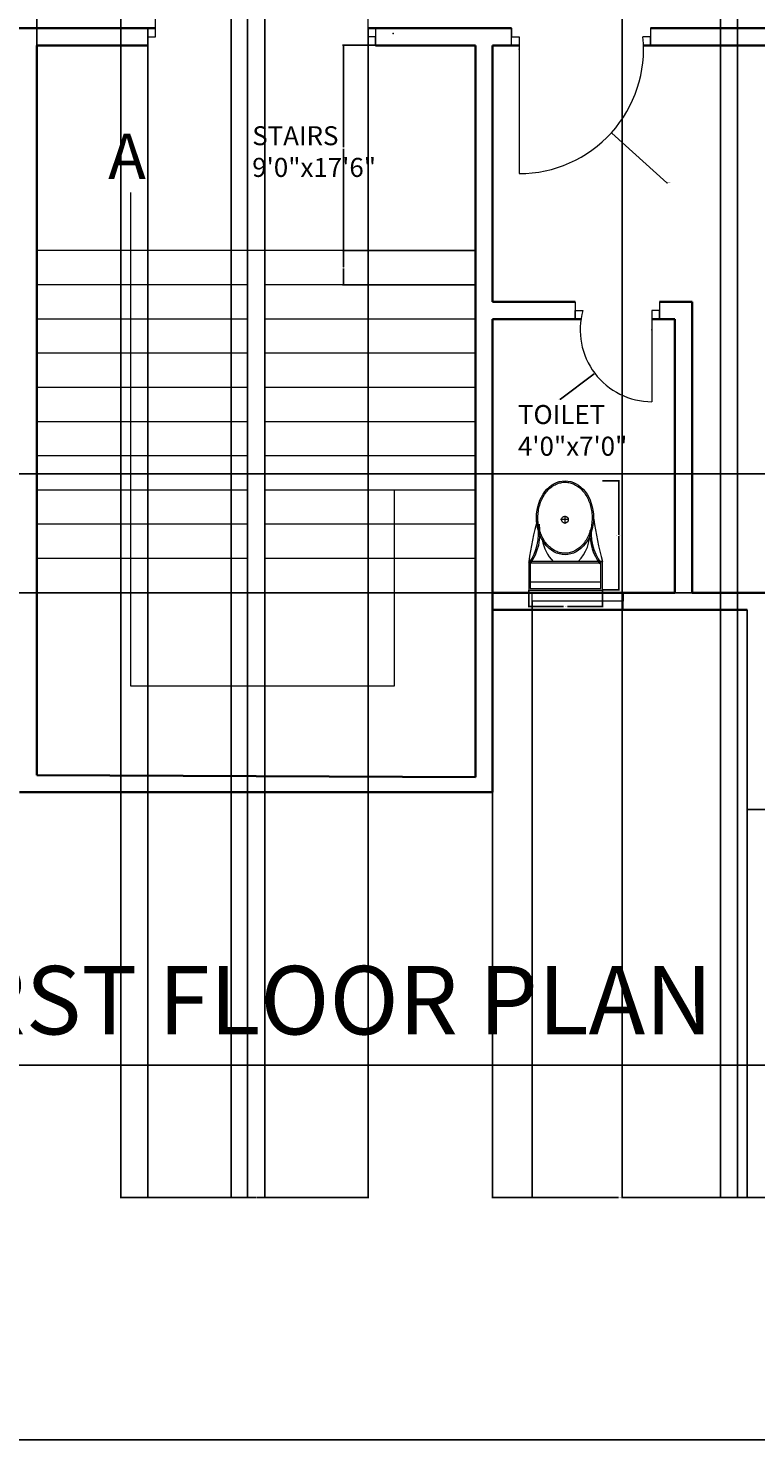
# Model space of a CAD drawing. Units: inches. Extents: x 1861 to 2564, y 1482 to 2317.
# Tile 2 of 11: x 2155 to 2347, y 1482 to 1853. Entities that reach past the tile are written whole.
import ezdxf

# ---------------------------------------------------------------- set-up
doc = ezdxf.new("R2010")
doc.units = ezdxf.units.IN
for name, color, linetype, lineweight in [('A-ANNO-DIMS', 2, 'Continuous', 18), ('A-ANNO-SYMB', 7, 'Continuous', 18), ('A-ANNO-TEXT', 7, 'Continuous', 25), ('A-ANNO-TTLB', 7, 'Continuous', 25), ('A-AREA-IDEN', 7, 'Continuous', 18), ('A-DOOR', 3, 'Continuous', 18), ('A-FLOR-EDGE', 7, 'Continuous', 25), ('A-FLOR-FIXT', 8, 'Continuous', 18), ('A-FLOR-STRS', 7, 'Continuous', 18), ('A-GLAZ', 4, 'Continuous', 18), ('A-WALL', 7, 'Continuous', 35)]:
    doc.layers.add(name, color=color, linetype=linetype, lineweight=lineweight)
doc.styles.get("Standard").update_dxf_attribs({"font": 'arial.ttf'})
doc.dimstyles.get("Standard").update_dxf_attribs({"dimtxt": 0.18, "dimasz": 0.18, "dimexe": 0.18, "dimexo": 0.0625, "dimgap": 0.09, "dimtad": 0, "dimtih": 1, "dimtoh": 1, "dimdec": 4, "dimzin": 0, "dimdsep": 46, "dimtxsty": 'Standard', "dimcen": 0.09, "dimadec": 0, "dimazin": 0, "dimtfac": 1, "dimtdec": 4, "dimtofl": 0, "dimtmove": 0, "dimatfit": 3, "dimfxl": 1, "dimtolj": 1, "dimtzin": 0, "dimarcsym": 0})

# ---------------------------------------------------------------- blocks, each defined once
blk = doc.blocks.new('A$C31115884')
for p, q in [((257.5, 466.4), (257.5, 523.2)), ((283.1, 497.7), (223.4, 497.7)), ((0, 200), (0, 0)), ((520, 200), (0, 200)), ((520, 0), (520, 200)), ((10, 190), (10, 10)), ((510, 190), (10, 190)), ((510, 10), (510, 190)), ((510, 54.5), (0, 54.5)), ((10, 10), (510, 10)), ((0, 0), (520, 0))]:
    blk.add_line(p, q)
blk.add_circle((255.6, 496.4), 23.6)
for centre, radius, start, end in [((2777.7, -204.6), 2807, 165.4549, 171.71327), ((3237, 905), 2807, 188.28673, 194.5451), ((-294.5, 403.3), 364.7, 324.20913, 9.34987), ((-294.5, 403.3), 374.7, 324.20913, 9.34987), ((139.5, 406.2), 293.5, 315.84364, 2.65635), ((805.8, 403.3), 374.7, 179.20365, 215.79087), ((805.8, 403.3), 364.7, 170.65013, 215.79087), ((383.6, 406.2), 293.5, 190.27735, 224.15636)]:
    blk.add_arc(centre, radius, start, end)
blk.add_ellipse((256.2, 509.9), major_axis=(0, -260.7), ratio=0.772727)
blk.add_open_spline([(256.2, 259.2), (263.1, 259.2), (270, 259.7), (287.8, 262.3), (298.7, 265.1), (319.9, 273.1), (330.2, 278.4), (350.1, 291.1), (359.7, 298.7), (377.7, 315.9), (386.2, 325.5), (401.7, 346.6), (408.8, 358.1), (421.3, 382.5), (426.8, 395.5), (435.9, 422.4), (439.5, 436.4), (444.8, 465.1), (446.5, 479.7), (447.9, 509.2), (447.6, 524), (445, 553.3), (442.7, 567.8), (436.3, 596), (432.1, 609.7), (421.9, 636), (416, 648.6), (402.5, 672.1), (395, 683), (378.6, 703), (369.8, 712.1), (351.1, 728), (341.3, 734.8), (320.9, 746.2), (310.4, 750.7), (288.9, 757.3), (278, 759.4), (256, 761), (245, 760.6), (223.1, 757.2), (212.3, 754.3), (191.1, 746.1), (180.8, 740.7), (160.9, 727.8), (151.4, 720.1), (133.5, 702.7), (125.1, 693), (109.6, 671.7), (102.6, 660.2), (90.2, 635.7), (84.9, 622.7), (76, 595.6), (72.4, 581.6), (67.2, 552.9), (65.6, 538.2), (64.4, 508.8), (64.8, 494), (67.5, 464.7), (69.9, 450.2), (76.6, 422), (80.8, 408.3), (91.1, 382.2), (97.2, 369.7), (110.8, 346.3), (118.4, 335.4), (134.8, 315.6), (143.7, 306.7), (162.4, 290.9), (172.3, 284.2), (192.8, 273), (203.3, 268.6), (224.8, 262.2), (235.8, 260.2), (249.9, 259.3), (253, 259.2), (256.2, 259.2)], degree=3, knots=[0, 0, 0, 0, 0.110105, 0.110105, 0.285049, 0.285049, 0.459994, 0.459994, 0.634938, 0.634938, 0.809882, 0.809882, 0.984827, 0.984827, 1.159771, 1.159771, 1.334715, 1.334715, 1.50966, 1.50966, 1.684604, 1.684604, 1.859549, 1.859549, 2.034493, 2.034493, 2.209437, 2.209437, 2.384382, 2.384382, 2.559326, 2.559326, 2.73427, 2.73427, 2.909215, 2.909215, 3.084159, 3.084159, 3.259103, 3.259103, 3.434048, 3.434048, 3.608992, 3.608992, 3.783936, 3.783936, 3.958881, 3.958881, 4.133825, 4.133825, 4.30877, 4.30877, 4.483714, 4.483714, 4.658658, 4.658658, 4.833603, 4.833603, 5.008547, 5.008547, 5.183491, 5.183491, 5.358436, 5.358436, 5.53338, 5.53338, 5.708324, 5.708324, 5.883269, 5.883269, 6.058213, 6.058213, 6.233158, 6.233158, 6.283185, 6.283185, 6.283185, 6.283185])
blk = doc.blocks.new('WIN-24IN')
for p, q in [((0, 24), (4.5, 24)), ((4.5, 24), (2.25, 24)), ((2.25, 24), (2.25, 0)), ((2.25, 0), (0, 0)), ((0, 0), (4.5, 0))]:
    blk.add_line(p, q)
blk = doc.blocks.new('*D14')
at = {"layer": 'A-ANNO-DIMS', "color": 0, "lineweight": -2, "transparency": 16777216}
for p, q in [((2306.19, 1734.33), (2310.61, 1734.33)), ((2310.43, 1734.15), (2310.43, 1720.15)), ((2310.43, 1705.79), (2310.43, 1719.79)), ((2306.19, 1705.61), (2310.61, 1705.61))]:
    blk.add_line(p, q, dxfattribs=at)
at = {"layer": 'A-ANNO-DIMS', "color": 0, "transparency": 16777216}
for points in [[(2310.4, 1734.15), (2310.46, 1734.15), (2310.43, 1734.33)], [(2310.4, 1705.79), (2310.46, 1705.79), (2310.43, 1705.61)]]:
    blk.add_solid(points, dxfattribs=at)
at = {"layer": 'Defpoints', "color": 0, "transparency": 16777216}
for p in [(2306.13, 1734.33), (2310.43, 1734.33), (2306.13, 1705.61)]:
    blk.add_point(p, dxfattribs=at)
at = {"layer": 'A-ANNO-DIMS', "color": 0, "transparency": 16777216, "insert": (2310.43, 1719.97), "char_height": 0.18, "attachment_point": 5}
blk.add_mtext('\\A1;WC 29 TYP.', dxfattribs=at)
blk = doc.blocks.new('*D15')
at = {"layer": 'A-ANNO-DIMS', "color": 0, "lineweight": -2, "transparency": 16777216}
for p, q in [((2286.74, 1705.55), (2286.74, 1701.12)), ((2306.13, 1705.55), (2306.13, 1701.12)), ((2286.92, 1701.3), (2295.92, 1701.3)), ((2305.95, 1701.3), (2296.96, 1701.3))]:
    blk.add_line(p, q, dxfattribs=at)
at = {"layer": 'A-ANNO-DIMS', "color": 0, "transparency": 16777216}
for points in [[(2286.92, 1701.33), (2286.92, 1701.27), (2286.74, 1701.3)], [(2305.95, 1701.33), (2305.95, 1701.27), (2306.13, 1701.3)]]:
    blk.add_solid(points, dxfattribs=at)
at = {"layer": 'Defpoints', "color": 0, "transparency": 16777216}
for p in [(2286.74, 1705.61), (2306.13, 1705.61), (2306.13, 1701.3)]:
    blk.add_point(p, dxfattribs=at)
at = {"layer": 'A-ANNO-DIMS', "color": 0, "transparency": 16777216, "insert": (2296.44, 1701.3), "char_height": 0.18, "attachment_point": 5}
blk.add_mtext('\\A1;19 TYP.', dxfattribs=at)
blk = doc.blocks.new('*D37')
at = {"layer": 'A-ANNO-DIMS', "color": 0, "lineweight": -2, "transparency": 16777216}
for p, q in [((2311.38, 2250.82), (2311.38, 1545.6)), ((2337.24, 2250.82), (2337.24, 1545.6)), ((2311.56, 1545.78), (2323.91, 1545.78)), ((2337.06, 1545.78), (2324.7, 1545.78))]:
    blk.add_line(p, q, dxfattribs=at)
at = {"layer": 'A-ANNO-DIMS', "color": 0, "transparency": 16777216}
for points in [[(2311.56, 1545.81), (2311.56, 1545.75), (2311.38, 1545.78)], [(2337.06, 1545.81), (2337.06, 1545.75), (2337.24, 1545.78)]]:
    blk.add_solid(points, dxfattribs=at)
at = {"layer": 'Defpoints', "color": 0, "transparency": 16777216}
for p in [(2311.38, 2250.89), (2337.24, 2250.89), (2337.24, 1545.78)]:
    blk.add_point(p, dxfattribs=at)
at = {"layer": 'A-ANNO-DIMS', "color": 0, "transparency": 16777216, "insert": (2324.31, 1545.78), "char_height": 0.18, "attachment_point": 5}
blk.add_mtext('\\A1;25.86', dxfattribs=at)
blk = doc.blocks.new('*D38')
at = {"layer": 'A-ANNO-DIMS', "color": 0, "lineweight": -2, "transparency": 16777216}
for p, q in [((2341.74, 2250.82), (2341.74, 1545.6)), ((2381.24, 2250.82), (2381.24, 1545.6)), ((2341.92, 1545.78), (2361.16, 1545.78)), ((2381.06, 1545.78), (2361.81, 1545.78))]:
    blk.add_line(p, q, dxfattribs=at)
at = {"layer": 'A-ANNO-DIMS', "color": 0, "transparency": 16777216}
for points in [[(2341.92, 1545.81), (2341.92, 1545.75), (2341.74, 1545.78)], [(2381.06, 1545.81), (2381.06, 1545.75), (2381.24, 1545.78)]]:
    blk.add_solid(points, dxfattribs=at)
at = {"layer": 'Defpoints', "color": 0, "transparency": 16777216}
for p in [(2341.74, 2250.89), (2381.24, 2250.89), (2381.24, 1545.78)]:
    blk.add_point(p, dxfattribs=at)
at = {"layer": 'A-ANNO-DIMS', "color": 0, "transparency": 16777216, "insert": (2361.49, 1545.78), "char_height": 0.18, "attachment_point": 5}
blk.add_mtext('\\A1;39.5', dxfattribs=at)
blk = doc.blocks.new('*D48')
at = {"layer": 'A-ANNO-DIMS', "color": 0, "lineweight": -2, "transparency": 16777216}
for p, q in [((2277.24, 1652.32), (2277.24, 1545.6)), ((2344.26, 1647.82), (2344.26, 1545.6)), ((2277.42, 1545.78), (2310.36, 1545.78)), ((2344.08, 1545.78), (2311.14, 1545.78))]:
    blk.add_line(p, q, dxfattribs=at)
at = {"layer": 'A-ANNO-DIMS', "color": 0, "transparency": 16777216}
for points in [[(2277.42, 1545.81), (2277.42, 1545.75), (2277.24, 1545.78)], [(2344.08, 1545.81), (2344.08, 1545.75), (2344.26, 1545.78)]]:
    blk.add_solid(points, dxfattribs=at)
at = {"layer": 'Defpoints', "color": 0, "transparency": 16777216}
for p in [(2277.24, 1652.39), (2344.26, 1647.89), (2344.26, 1545.78)]:
    blk.add_point(p, dxfattribs=at)
at = {"layer": 'A-ANNO-DIMS', "color": 0, "transparency": 16777216, "insert": (2310.75, 1545.78), "char_height": 0.18, "attachment_point": 5}
blk.add_mtext('\\A1;67.02', dxfattribs=at)
blk = doc.blocks.new('*D52')
at = {"layer": 'A-ANNO-DIMS', "color": 0, "lineweight": -2, "transparency": 16777216}
for p, q in [((2179.39, 2154.82), (2179.39, 1545.6)), ((2208.37, 2154.82), (2208.37, 1545.6)), ((2179.57, 1545.78), (2193.49, 1545.78)), ((2208.19, 1545.78), (2194.28, 1545.78))]:
    blk.add_line(p, q, dxfattribs=at)
at = {"layer": 'A-ANNO-DIMS', "color": 0, "transparency": 16777216}
for points in [[(2179.57, 1545.81), (2179.57, 1545.75), (2179.39, 1545.78)], [(2208.19, 1545.81), (2208.19, 1545.75), (2208.37, 1545.78)]]:
    blk.add_solid(points, dxfattribs=at)
at = {"layer": 'Defpoints', "color": 0, "transparency": 16777216}
for p in [(2179.39, 2154.89), (2208.37, 2154.89), (2208.37, 1545.78)]:
    blk.add_point(p, dxfattribs=at)
at = {"layer": 'A-ANNO-DIMS', "color": 0, "transparency": 16777216, "insert": (2193.88, 1545.78), "char_height": 0.18, "attachment_point": 5}
blk.add_mtext('\\A1;28.98', dxfattribs=at)
blk = doc.blocks.new('*D56')
at = {"layer": 'A-ANNO-DIMS', "color": 0, "lineweight": -2, "transparency": 16777216}
for p, q in [((2186.51, 1853.32), (2186.51, 1545.6)), ((2244.44, 1853.32), (2244.44, 1545.6)), ((2186.69, 1545.78), (2215.08, 1545.78)), ((2244.26, 1545.78), (2215.87, 1545.78))]:
    blk.add_line(p, q, dxfattribs=at)
at = {"layer": 'A-ANNO-DIMS', "color": 0, "transparency": 16777216}
for points in [[(2186.69, 1545.81), (2186.69, 1545.75), (2186.51, 1545.78)], [(2244.26, 1545.81), (2244.26, 1545.75), (2244.44, 1545.78)]]:
    blk.add_solid(points, dxfattribs=at)
at = {"layer": 'Defpoints', "color": 0, "transparency": 16777216}
for p in [(2186.51, 1853.39), (2244.44, 1853.39), (2244.44, 1545.78)]:
    blk.add_point(p, dxfattribs=at)
at = {"layer": 'A-ANNO-DIMS', "color": 0, "transparency": 16777216, "insert": (2215.48, 1545.78), "char_height": 0.18, "attachment_point": 5}
blk.add_mtext('\\A1;57.93', dxfattribs=at)
blk = doc.blocks.new('*D67')
at = {"layer": 'A-ANNO-DIMS', "color": 0, "lineweight": -2, "transparency": 16777216}
for p, q in [((2497.68, 1736.13), (1892.76, 1736.13)), ((1892.94, 1735.95), (1892.94, 1720.69)), ((1892.94, 1705.07), (1892.94, 1720.32)), ((2497.68, 1704.89), (1892.76, 1704.89))]:
    blk.add_line(p, q, dxfattribs=at)
at = {"layer": 'A-ANNO-DIMS', "color": 0, "transparency": 16777216}
for points in [[(1892.91, 1735.95), (1892.97, 1735.95), (1892.94, 1736.13)], [(1892.91, 1705.07), (1892.97, 1705.07), (1892.94, 1704.89)]]:
    blk.add_solid(points, dxfattribs=at)
at = {"layer": 'Defpoints', "color": 0, "transparency": 16777216}
for p in [(1892.94, 1736.13), (2497.74, 1736.13), (2497.74, 1704.89)]:
    blk.add_point(p, dxfattribs=at)
at = {"layer": 'A-ANNO-DIMS', "color": 0, "transparency": 16777216, "insert": (1892.94, 1720.51), "char_height": 0.18, "attachment_point": 5}
blk.add_mtext('\\A1;31.24', dxfattribs=at)
blk = doc.blocks.new('*D68')
at = {"layer": 'A-ANNO-DIMS', "color": 0, "lineweight": -2, "transparency": 16777216}
for p, q in [((2157.24, 1794.95), (2157.24, 2290.37)), ((2157.42, 2290.19), (2184.66, 2290.19)), ((2212.56, 2290.19), (2185.31, 2290.19)), ((2212.74, 1794.95), (2212.74, 2290.37))]:
    blk.add_line(p, q, dxfattribs=at)
at = {"layer": 'A-ANNO-DIMS', "color": 0, "transparency": 16777216}
for points in [[(2157.42, 2290.22), (2157.42, 2290.16), (2157.24, 2290.19)], [(2212.56, 2290.22), (2212.56, 2290.16), (2212.74, 2290.19)]]:
    blk.add_solid(points, dxfattribs=at)
at = {"layer": 'Defpoints', "color": 0, "transparency": 16777216}
for p in [(2212.74, 2290.19), (2157.24, 1794.89), (2212.74, 1794.89)]:
    blk.add_point(p, dxfattribs=at)
at = {"layer": 'A-ANNO-DIMS', "color": 0, "transparency": 16777216, "insert": (2184.99, 2290.19), "char_height": 0.18, "attachment_point": 5}
blk.add_mtext('\\A1;55.5', dxfattribs=at)
blk = doc.blocks.new('*D69')
at = {"layer": 'A-ANNO-DIMS', "color": 0, "lineweight": -2, "transparency": 16777216}
for p, q in [((2272.68, 1794.89), (2237.76, 1794.89)), ((2237.94, 1794.71), (2237.94, 1790.57)), ((2237.94, 1786.07), (2237.94, 1790.2)), ((2272.68, 1785.89), (2237.76, 1785.89))]:
    blk.add_line(p, q, dxfattribs=at)
at = {"layer": 'A-ANNO-DIMS', "color": 0, "transparency": 16777216}
for points in [[(2237.91, 1794.71), (2237.97, 1794.71), (2237.94, 1794.89)], [(2237.91, 1786.07), (2237.97, 1786.07), (2237.94, 1785.89)]]:
    blk.add_solid(points, dxfattribs=at)
at = {"layer": 'Defpoints', "color": 0, "transparency": 16777216}
for p in [(2237.94, 1794.89), (2272.74, 1794.89), (2272.74, 1785.89)]:
    blk.add_point(p, dxfattribs=at)
at = {"layer": 'A-ANNO-DIMS', "color": 0, "transparency": 16777216, "insert": (2237.94, 1790.39), "char_height": 0.18, "attachment_point": 5}
blk.add_mtext('\\A1;9', dxfattribs=at)
blk = doc.blocks.new('*D70')
at = {"layer": 'A-ANNO-DIMS', "color": 0, "lineweight": -2, "transparency": 16777216}
for p, q in [((2272.68, 1848.89), (2237.76, 1848.89)), ((2237.94, 1848.71), (2237.94, 1822.07)), ((2237.94, 1795.07), (2237.94, 1821.7)), ((2272.68, 1794.89), (2237.76, 1794.89))]:
    blk.add_line(p, q, dxfattribs=at)
at = {"layer": 'A-ANNO-DIMS', "color": 0, "transparency": 16777216}
for points in [[(2237.91, 1848.71), (2237.97, 1848.71), (2237.94, 1848.89)], [(2237.91, 1795.07), (2237.97, 1795.07), (2237.94, 1794.89)]]:
    blk.add_solid(points, dxfattribs=at)
at = {"layer": 'Defpoints', "color": 0, "transparency": 16777216}
for p in [(2237.94, 1848.89), (2272.74, 1848.89), (2272.74, 1794.89)]:
    blk.add_point(p, dxfattribs=at)
at = {"layer": 'A-ANNO-DIMS', "color": 0, "transparency": 16777216, "insert": (2237.94, 1821.89), "char_height": 0.18, "attachment_point": 5}
blk.add_mtext('\\A1;54', dxfattribs=at)
blk = doc.blocks.new('*D71')
at = {"layer": 'A-ANNO-DIMS', "color": 0, "lineweight": -2, "transparency": 16777216}
for p, q in [((2212.74, 2250.82), (2212.74, 1545.6)), ((2217.24, 2250.82), (2217.24, 1545.6)), ((2212.92, 1545.78), (2214.73, 1545.78)), ((2217.06, 1545.78), (2215.25, 1545.78))]:
    blk.add_line(p, q, dxfattribs=at)
at = {"layer": 'A-ANNO-DIMS', "color": 0, "transparency": 16777216}
for points in [[(2212.92, 1545.81), (2212.92, 1545.75), (2212.74, 1545.78)], [(2217.06, 1545.81), (2217.06, 1545.75), (2217.24, 1545.78)]]:
    blk.add_solid(points, dxfattribs=at)
at = {"layer": 'Defpoints', "color": 0, "transparency": 16777216}
for p in [(2212.74, 2250.89), (2217.24, 2250.89), (2217.24, 1545.78)]:
    blk.add_point(p, dxfattribs=at)
at = {"layer": 'A-ANNO-DIMS', "color": 0, "transparency": 16777216, "insert": (2214.99, 1545.78), "char_height": 0.18, "attachment_point": 5}
blk.add_mtext('\\A1;4.5', dxfattribs=at)
blk = doc.blocks.new('*D73')
at = {"layer": 'A-ANNO-DIMS', "color": 0, "lineweight": -2, "transparency": 16777216}
for p, q in [((2277.24, 1700.32), (2277.24, 1545.6)), ((2287.62, 1700.32), (2287.62, 1545.6)), ((2277.42, 1545.78), (2281.98, 1545.78)), ((2287.44, 1545.78), (2282.89, 1545.78))]:
    blk.add_line(p, q, dxfattribs=at)
at = {"layer": 'A-ANNO-DIMS', "color": 0, "transparency": 16777216}
for points in [[(2277.42, 1545.81), (2277.42, 1545.75), (2277.24, 1545.78)], [(2287.44, 1545.81), (2287.44, 1545.75), (2287.62, 1545.78)]]:
    blk.add_solid(points, dxfattribs=at)
at = {"layer": 'Defpoints', "color": 0, "transparency": 16777216}
for p in [(2277.24, 1700.39), (2287.62, 1700.39), (2287.62, 1545.78)]:
    blk.add_point(p, dxfattribs=at)
at = {"layer": 'A-ANNO-DIMS', "color": 0, "transparency": 16777216, "insert": (2282.43, 1545.78), "char_height": 0.18, "attachment_point": 5}
blk.add_mtext('\\A1;10.383', dxfattribs=at)
blk = doc.blocks.new('*D74')
at = {"layer": 'A-ANNO-DIMS', "color": 0, "lineweight": -2, "transparency": 16777216}
for p, q in [((2212.63, 1894.56), (2212.81, 1894.56)), ((2212.81, 1894.56), (2227.02, 1878.73)), ((2250.93, 1852), (2251.11, 1852)), ((2251.02, 1851.91), (2251.02, 1852.09))]:
    blk.add_line(p, q, dxfattribs=at)
at = {"layer": 'A-ANNO-DIMS', "color": 0, "transparency": 16777216}
blk.add_solid([(2227.04, 1878.75), (2227, 1878.71), (2227.14, 1878.6)], dxfattribs=at)
at = {"layer": 'Defpoints', "color": 0, "transparency": 16777216}
for p in [(2227.14, 1878.6), (2251.02, 1852)]:
    blk.add_point(p, dxfattribs=at)
at = {"layer": 'A-ANNO-DIMS', "color": 0, "transparency": 16777216, "insert": (2212.16, 1894.56), "char_height": 0.18, "attachment_point": 5}
blk.add_mtext('\\A1;R35.74', dxfattribs=at)
blk = doc.blocks.new('*D75')
at = {"layer": 'A-ANNO-DIMS', "color": 0, "lineweight": -2, "transparency": 16777216}
for p, q in [((2284.14, 1847.87), (2284.32, 1847.87)), ((2284.23, 1847.78), (2284.23, 1847.96)), ((2323.07, 1812.73), (2308.64, 1825.79)), ((2323.25, 1812.73), (2323.07, 1812.73))]:
    blk.add_line(p, q, dxfattribs=at)
at = {"layer": 'A-ANNO-DIMS', "color": 0, "transparency": 16777216}
blk.add_solid([(2308.66, 1825.81), (2308.62, 1825.76), (2308.5, 1825.91)], dxfattribs=at)
at = {"layer": 'Defpoints', "color": 0, "transparency": 16777216}
for p in [(2284.23, 1847.87), (2308.5, 1825.91)]:
    blk.add_point(p, dxfattribs=at)
at = {"layer": 'A-ANNO-DIMS', "color": 0, "transparency": 16777216, "insert": (2323.73, 1812.73), "char_height": 0.18, "attachment_point": 5}
blk.add_mtext('\\A1;R32.74', dxfattribs=at)
blk = doc.blocks.new('*D89')
at = {"layer": 'A-ANNO-DIMS', "color": 0, "lineweight": -2, "transparency": 16777216}
for p, q in [((2319.07, 1774.01), (2319.25, 1774.01)), ((2319.16, 1773.92), (2319.16, 1774.1)), ((2295.08, 1755.78), (2303.96, 1762.51)), ((2294.9, 1755.78), (2295.08, 1755.78))]:
    blk.add_line(p, q, dxfattribs=at)
at = {"layer": 'A-ANNO-DIMS', "color": 0, "transparency": 16777216}
blk.add_solid([(2303.95, 1762.53), (2303.98, 1762.49), (2304.11, 1762.62)], dxfattribs=at)
at = {"layer": 'Defpoints', "color": 0, "transparency": 16777216}
for p in [(2319.16, 1774.01), (2304.11, 1762.62)]:
    blk.add_point(p, dxfattribs=at)
at = {"layer": 'A-ANNO-DIMS', "color": 0, "transparency": 16777216, "insert": (2294.42, 1755.78), "char_height": 0.18, "attachment_point": 5}
blk.add_mtext('\\A1;R18.88', dxfattribs=at)

msp = doc.modelspace()

# ---------------------------------------------------------------- linework, layer by layer
at = {"layer": 'A-ANNO-TTLB'}
msp.add_line((2110.0229, 1580.5777), (2362.3195, 1580.5777), dxfattribs=at)
msp.add_lwpolyline([(1861.1332, 2316.6589), (2563.8077, 2316.6589), (2563.8077, 1482.0728), (1861.1332, 1482.0728)], close=True, dxfattribs=at)
at = {"layer": 'A-DOOR'}
for p, q in [((2188.5091, 1851.1354), (2188.5091, 1887.1354)), ((2244.4436, 1851.1354), (2244.4436, 1887.1354)), ((2186.5091, 1853.3854), (2186.5091, 1848.8854)), ((2246.4436, 1853.3854), (2246.4436, 1848.8854)), ((2282.2262, 1848.8854), (2282.2262, 1853.3854)), ((2282.2262, 1853.3854), (2282.2262, 1851.1354)), ((2318.8029, 1853.3854), (2318.8029, 1848.8854)), ((2186.5091, 1848.8854), (2186.5091, 1851.1354)), ((2186.5091, 1851.1354), (2188.5091, 1851.1354)), ((2246.4436, 1851.1354), (2244.4436, 1851.1354)), ((2246.4436, 1848.8854), (2246.4436, 1851.1354)), ((2282.2262, 1851.1354), (2284.2262, 1851.1354)), ((2284.2262, 1851.1354), (2284.2262, 1815.1354)), ((2318.8029, 1851.1354), (2316.8029, 1851.1354)), ((2318.8029, 1848.8854), (2318.8029, 1851.1354)), ((2298.9893, 1781.3854), (2298.9893, 1776.8854)), ((2298.9893, 1776.8854), (2298.9893, 1779.1354)), ((2298.9893, 1779.1354), (2300.9893, 1779.1354)), ((2321.1596, 1779.1354), (2319.1596, 1779.1354)), ((2319.1596, 1779.1354), (2319.1596, 1755.1354)), ((2321.1596, 1781.3854), (2321.1596, 1776.8854)), ((2321.1596, 1776.8854), (2321.1596, 1779.1354))]:
    msp.add_line(p, q, dxfattribs=at)
for centre, radius, start, end in [((2284.2262, 1847.8749), 32.7395, 270, 5.715545), ((2319.1596, 1774.0137), 18.8783, 164.25844, 270)]:
    msp.add_arc(centre, radius, start, end, dxfattribs=at)
at = {"layer": 'A-FLOR-EDGE'}
for p, q in [((2344.2613, 1700.3854), (2344.2613, 1647.8854)), ((2344.2613, 1647.8854), (2468.7613, 1647.8854))]:
    msp.add_line(p, q, dxfattribs=at)
at = {"layer": 'A-FLOR-STRS'}
for p, q in [((2181.9292, 1810.1769), (2181.9292, 1680.3574)), ((2272.7393, 1794.8854), (2157.2393, 1794.8854)), ((2212.7393, 1794.8854), (2212.7393, 1704.8854)), ((2217.2393, 1794.8854), (2217.2393, 1704.8854)), ((2212.7393, 1785.8854), (2157.2393, 1785.8854)), ((2272.7393, 1785.8854), (2217.2393, 1785.8854)), ((2212.7393, 1776.8854), (2157.2393, 1776.8854)), ((2272.7393, 1776.8854), (2217.2393, 1776.8854)), ((2212.7393, 1767.8854), (2157.2393, 1767.8854)), ((2272.7393, 1767.8854), (2217.2393, 1767.8854)), ((2212.7393, 1758.8854), (2157.2393, 1758.8854)), ((2272.7393, 1758.8854), (2217.2393, 1758.8854)), ((2212.7393, 1749.8854), (2157.2393, 1749.8854)), ((2272.7393, 1749.8854), (2217.2393, 1749.8854)), ((2212.7393, 1740.8854), (2157.2393, 1740.8854)), ((2272.7393, 1740.8854), (2217.2393, 1740.8854)), ((2212.7393, 1731.8854), (2157.2393, 1731.8854)), ((2272.7393, 1731.8854), (2217.2393, 1731.8854)), ((2251.4277, 1680.3574), (2251.4277, 1731.8854)), ((2212.7393, 1722.8854), (2157.2393, 1722.8854)), ((2272.7393, 1722.8854), (2217.2393, 1722.8854)), ((2212.7393, 1713.8854), (2157.2393, 1713.8854)), ((2272.7393, 1713.8854), (2217.2393, 1713.8854)), ((2272.7393, 1704.8854), (2157.2393, 1704.8854)), ((2272.7393, 1704.8854), (2217.2393, 1704.8854)), ((2181.9292, 1680.3574), (2251.4277, 1680.3574))]:
    msp.add_line(p, q, dxfattribs=at)
at = {"layer": 'A-WALL'}
for p, q in [((2188.5091, 1853.3854), (2146.7425, 1853.3854)), ((2282.2262, 1853.3854), (2244.4436, 1853.3854)), ((2421.2393, 1853.3854), (2318.8029, 1853.3854)), ((2157.2393, 1704.8854), (2157.2393, 1848.8854)), ((2157.2393, 1848.8854), (2186.5091, 1848.8854)), ((2246.4436, 1848.8854), (2272.7393, 1848.8854)), ((2272.7393, 1848.8854), (2272.7393, 1704.8854)), ((2277.2393, 1848.8854), (2284.2262, 1848.8854)), ((2277.2393, 1781.3854), (2277.2393, 1848.8854)), ((2316.9501, 1848.8854), (2497.7393, 1848.8854)), ((2497.7393, 1848.8854), (2329.7393, 1848.8854)), ((2272.7393, 1781.3854), (2272.7393, 1776.8854)), ((2298.9893, 1781.3854), (2277.2393, 1781.3854)), ((2329.7393, 1781.3854), (2321.1596, 1781.3854)), ((2329.7393, 1781.3854), (2329.7393, 1704.8854)), ((2277.2393, 1704.8854), (2277.2393, 1776.8854)), ((2277.2393, 1776.8854), (2300.5009, 1776.8854)), ((2319.1596, 1776.8854), (2325.2393, 1776.8854)), ((2325.2393, 1704.8854), (2325.2393, 1776.8854)), ((2157.2393, 1704.8854), (2157.2393, 1656.8854)), ((2272.7393, 1704.8854), (2272.7393, 1656.3854)), ((2325.2393, 1704.8854), (2277.2393, 1704.8854)), ((2277.2393, 1652.3854), (2277.2393, 1704.8854)), ((2325.2393, 1704.8854), (2277.2393, 1704.8854)), ((2356.0129, 1704.8854), (2329.7393, 1704.8854)), ((2277.2393, 1700.3854), (2344.2613, 1700.3854)), ((2157.2393, 1656.8854), (2272.7393, 1656.3854)), ((2152.7393, 1652.3854), (2277.2393, 1652.3854))]:
    msp.add_line(p, q, dxfattribs=at)

# ---------------------------------------------------------------- block references
at = {"layer": 'A-FLOR-FIXT', "xscale": 0.0372717239612423, "yscale": 0.0372717239612423, "zscale": 0.0372717239612423}
msp.add_blockref('A$C31115884', (2286.745, 1705.6086), dxfattribs=at)
at = {"layer": 'A-GLAZ', "extrusion": (0, 0, -1), "zscale": -1, "rotation": 90}
msp.add_blockref('WIN-24IN', (-2287.6252, 1700.3861), dxfattribs=at)

# ---------------------------------------------------------------- texts
at = {"layer": 'A-ANNO-SYMB', "insert": (2176.0127, 1825.6922), "char_height": 12, "attachment_point": 1}
msp.add_mtext_dynamic_manual_height_columns('A', width=11.368027, gutter_width=12.5, heights=[0], dxfattribs=at)
at = {"layer": 'A-ANNO-TEXT', "insert": (2117.9934, 1606.7084), "char_height": 18, "attachment_point": 1}
msp.add_mtext_dynamic_manual_height_columns('FIRST FLOOR PLAN', width=523.098946, gutter_width=12.5, heights=[0], dxfattribs=at)
at = {"layer": 'A-AREA-IDEN', "char_height": 5, "attachment_point": 1}
for s, width, insert in [('STAIRS\\P9\'0"x17\'6"', 87.13383, (2213.9583, 1827.6097)), ('TOILET\\P4\'0"x7\'0"', 61.945432, (2283.9065, 1754.2671))]:
    msp.add_mtext_dynamic_manual_height_columns(s, width=width, gutter_width=12.5, heights=[0], dxfattribs=dict(at, insert=insert))

# ---------------------------------------------------------------- dimensions: what is measured, and where the dimension line sits
at = {"layer": 'A-ANNO-DIMS'}
for base, p1, p2, override, picture, middle in [((2212.7393, 2290.1854), (2157.2393, 1794.8854), (2212.7393, 1794.8854), {"dimdec": 1, "dimlfac": 1, "dimrnd": 0, "dimzin": 0, "dimdsep": 46, "dimlunit": 2}, '*D68', (2184.9893, 2290.1854)), ((2217.2393, 1545.7777), (2212.7393, 2250.8854), (2217.2393, 2250.8854), {"dimdec": 1, "dimlfac": 1, "dimrnd": 0, "dimzin": 0, "dimdsep": 46, "dimlunit": 2}, '*D71', (2214.9893, 1545.7777)), ((2337.2393, 1545.7777), (2311.3789, 2250.8854), (2337.2393, 2250.8854), {"dimdec": 2, "dimlfac": 1, "dimrnd": 0, "dimzin": 0, "dimdsep": 46, "dimlunit": 2}, '*D37', (2324.3091, 1545.7777)), ((2381.2368, 1545.7777), (2341.7393, 2250.8854), (2381.2368, 2250.8854), {"dimdec": 1, "dimlfac": 1, "dimrnd": 0, "dimzin": 0, "dimdsep": 46, "dimlunit": 2}, '*D38', (2361.488, 1545.7777)), ((2208.3728, 1545.7777), (2179.3907, 2154.8854), (2208.3728, 2154.8854), {"dimdec": 2, "dimlfac": 1, "dimrnd": 0, "dimzin": 0, "dimdsep": 46, "dimlunit": 2}, '*D52', (2193.8817, 1545.7777)), ((2244.4436, 1545.7777), (2186.5091, 1853.3854), (2244.4436, 1853.3854), {"dimdec": 2, "dimlfac": 1, "dimrnd": 0, "dimzin": 0, "dimdsep": 46, "dimlunit": 2}, '*D56', (2215.4763, 1545.7777)), ((2287.6222, 1545.7777), (2277.2393, 1700.3854), (2287.6222, 1700.3854), {"dimdec": 3, "dimlfac": 1, "dimrnd": 0, "dimzin": 0, "dimdsep": 46, "dimlunit": 2}, '*D73', (2282.4307, 1545.7777)), ((2344.2613, 1545.7777), (2277.2393, 1652.3854), (2344.2613, 1647.8854), {"dimdec": 2, "dimlfac": 1, "dimrnd": 0, "dimzin": 0, "dimdsep": 46, "dimlunit": 2}, '*D48', (2310.7503, 1545.7777))]:
    dim = msp.add_linear_dim(base=base, p1=p1, p2=p2, dimstyle='Standard', override=override, dxfattribs=at)
    dim.commit()
    dim.dimension.update_dxf_attribs({"geometry": picture, "text_midpoint": middle})
for center, mpoint, picture, middle in [((2251.0211, 1852.0028), (2227.1421, 1878.5989), '*D74', (2212.1552, 1894.5566)), ((2284.2262, 1847.8749), (2308.5022, 1825.9079), '*D75', (2323.7272, 1812.7276)), ((2319.1596, 1774.0137), (2304.1084, 1762.6183), '*D89', (2294.4177, 1755.7811))]:
    dim = msp.add_radius_dim(center=center, mpoint=mpoint, dimstyle='Standard', override={"dimdec": 2, "dimlfac": 1, "dimrnd": 0, "dimzin": 0, "dimdsep": 46, "dimlunit": 2}, dxfattribs=at)
    dim.commit()
    dim.dimension.update_dxf_attribs({"geometry": picture, "text_midpoint": middle, "dimtype": 164})
for base, p1, p2, override, picture, middle in [((2237.9393, 1848.8854), (2272.7393, 1794.8854), (2272.7393, 1848.8854), {"dimdec": 0, "dimlfac": 1, "dimrnd": 0, "dimzin": 0, "dimdsep": 46, "dimlunit": 2}, '*D70', (2237.9393, 1821.8854)), ((2237.9393, 1794.8854), (2272.7393, 1785.8854), (2272.7393, 1794.8854), {"dimdec": 0, "dimlfac": 1, "dimrnd": 0, "dimzin": 0, "dimdsep": 46, "dimlunit": 2}, '*D69', (2237.9393, 1790.3854)), ((1892.9393, 1736.1256), (2497.7393, 1704.8854), (2497.7393, 1736.1256), {"dimdec": 2, "dimlfac": 1, "dimrnd": 0, "dimzin": 0, "dimdsep": 46, "dimlunit": 2}, '*D67', (1892.9393, 1720.5055))]:
    dim = msp.add_linear_dim(base=base, p1=p1, p2=p2, angle=90, dimstyle='Standard', override=override, dxfattribs=at)
    dim.commit()
    dim.dimension.update_dxf_attribs({"geometry": picture, "text_midpoint": middle})
dim = msp.add_linear_dim(base=(2310.4344, 1734.3291), p1=(2306.1263, 1705.6086), p2=(2306.1263, 1734.3291), angle=90, text='WC <> TYP.', dimstyle='Standard', override={"dimdec": 0, "dimlfac": 1, "dimrnd": 0, "dimzin": 0, "dimdsep": 46, "dimlunit": 2}, dxfattribs=at)
dim.commit()
dim.dimension.update_dxf_attribs({"geometry": '*D14', "text_midpoint": (2310.4344, 1719.9689)})
dim = msp.add_linear_dim(base=(2306.1263, 1701.3006), p1=(2286.745, 1705.6086), p2=(2306.1263, 1705.6086), text='<> TYP.', dimstyle='Standard', override={"dimdec": 0, "dimlfac": 1, "dimrnd": 0, "dimzin": 0, "dimdsep": 46, "dimlunit": 2}, dxfattribs=at)
dim.commit()
dim.dimension.update_dxf_attribs({"geometry": '*D15', "text_midpoint": (2296.4356, 1701.3006)})

doc.saveas('drawing.dxf')
